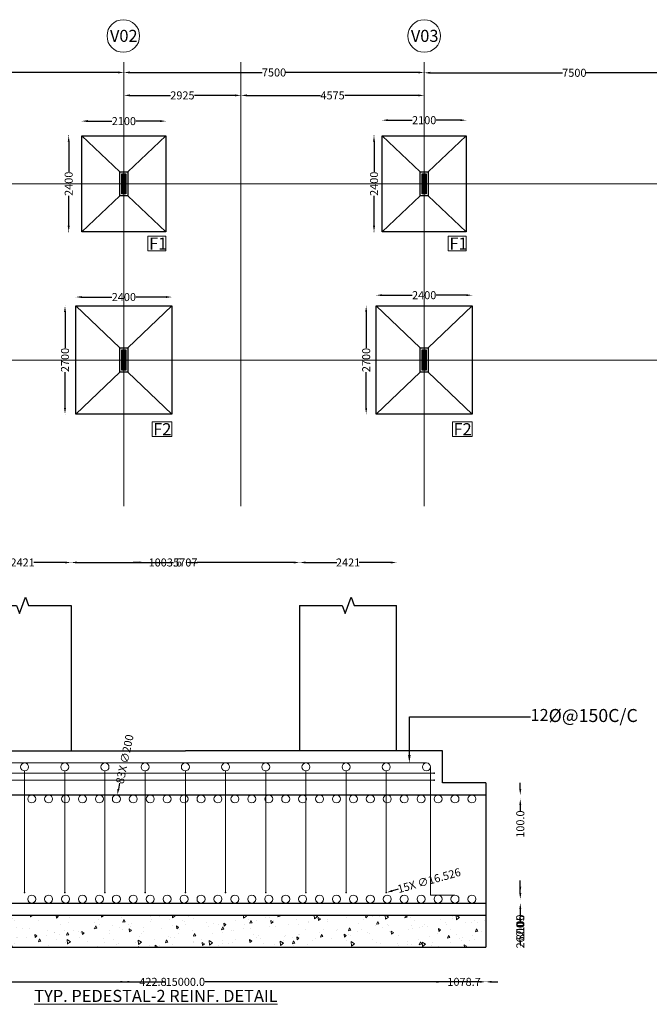
# Model space of a CAD drawing. Units: millimetres. Extents: x -30630 to 20484, y 3580 to 30715.
# Tile 2 of 4: x -19082 to -3358, y 3580 to 28161. Entities that reach past the tile are written whole.
import ezdxf
from ezdxf import colors
from ezdxf.entities.mleader import LeaderData, LeaderLine
from ezdxf.math import Vec2, Vec3

# ---------------------------------------------------------------- set-up
doc = ezdxf.new("R2010")
doc.units = ezdxf.units.MM
doc.header["$MEASUREMENT"] = 0
for name, color, linetype, lineweight in [('S-ANNO-DIMS', 2, 'Continuous', 18), ('S-ANNO-SYMB', 3, 'Continuous', 18), ('S-ANNO-TEXT', 7, 'Continuous', 18), ('S-CONC', 7, 'Continuous', 25), ('S-FNDN', 7, 'Continuous', 30), ('S-FNDN-PATT', 8, 'Continuous', 13), ('S-GRID', 1, 'Continuous', 18), ('S-GRID-IDEN', 7, 'Continuous', 18), ('S-REIN', 1, 'Continuous', 18)]:
    doc.layers.add(name, color=color, linetype=linetype, lineweight=lineweight)
doc.styles.get("Standard").update_dxf_attribs({"font": 'arial.ttf'})
doc.dimstyles.get("Standard").update_dxf_attribs({"dimtxt": 200, "dimasz": 150, "dimexe": 0.18, "dimexo": 0.0625, "dimgap": 0.09, "dimtad": 0, "dimdec": 0, "dimzin": 0, "dimdsep": 46, "dimtxsty": 'Standard', "dimcen": 0.09, "dimadec": 0, "dimazin": 0, "dimtfac": 1, "dimtdec": 0, "dimtofl": 0, "dimtmove": 0, "dimatfit": 3, "dimfxl": 1, "dimfxlon": 1, "dimtolj": 1, "dimtzin": 0, "dimarcsym": 0})

# ---------------------------------------------------------------- blocks, each defined once
blk = doc.blocks.new('*D1')
at = {"layer": 'Defpoints', "color": 0, "transparency": 16777216}
for p in [(-16480, 26844), (-23980, 25951), (-16480, 25951)]:
    blk.add_point(p, dxfattribs=at)
at = {"layer": 'S-ANNO-DIMS', "color": 0, "lineweight": -2, "transparency": 16777216}
for p, q in [((-23980, 26843), (-23980, 26844)), ((-23830, 26844), (-20528, 26844)), ((-16630, 26844), (-19933, 26844)), ((-16480, 26843), (-16480, 26844))]:
    blk.add_line(p, q, dxfattribs=at)
at = {"layer": 'S-ANNO-DIMS', "color": 0, "transparency": 16777216}
for points in [[(-23830, 26869), (-23830, 26819), (-23980, 26844)], [(-16630, 26869), (-16630, 26819), (-16480, 26844)]]:
    blk.add_solid(points, dxfattribs=at)
at = {"layer": 'S-ANNO-DIMS', "color": 0, "transparency": 16777216, "insert": (-20230, 26844), "char_height": 200, "attachment_point": 5}
blk.add_mtext('\\A1;7500', dxfattribs=at)
blk = doc.blocks.new('*D2')
at = {"layer": 'Defpoints', "color": 0, "transparency": 16777216}
for p in [(-16480, 26234), (-13555, 26271), (-13555, 26234)]:
    blk.add_point(p, dxfattribs=at)
at = {"layer": 'S-ANNO-DIMS', "color": 0, "lineweight": -2, "transparency": 16777216}
for p, q in [((-16480, 26270), (-16480, 26272)), ((-16330, 26271), (-15319, 26271)), ((-13705, 26271), (-14716, 26271)), ((-13555, 26270), (-13555, 26272))]:
    blk.add_line(p, q, dxfattribs=at)
at = {"layer": 'S-ANNO-DIMS', "color": 0, "transparency": 16777216}
for points in [[(-16330, 26296), (-16330, 26246), (-16480, 26271)], [(-13705, 26296), (-13705, 26246), (-13555, 26271)]]:
    blk.add_solid(points, dxfattribs=at)
at = {"layer": 'S-ANNO-DIMS', "color": 0, "transparency": 16777216, "insert": (-15018, 26271), "char_height": 200, "attachment_point": 5}
blk.add_mtext('\\A1;2925', dxfattribs=at)
blk = doc.blocks.new('*D3')
at = {"layer": 'Defpoints', "color": 0, "transparency": 16777216}
for p in [(-13555, 26271), (-8980, 26271), (-8980, 26271)]:
    blk.add_point(p, dxfattribs=at)
at = {"layer": 'S-ANNO-DIMS', "color": 0, "lineweight": -2, "transparency": 16777216}
for p, q in [((-13555, 26271), (-13555, 26271)), ((-13405, 26271), (-11571, 26271)), ((-9130, 26271), (-10964, 26271)), ((-8980, 26271), (-8980, 26271))]:
    blk.add_line(p, q, dxfattribs=at)
at = {"layer": 'S-ANNO-DIMS', "color": 0, "transparency": 16777216}
for points in [[(-13405, 26296), (-13405, 26246), (-13555, 26271)], [(-9130, 26296), (-9130, 26246), (-8980, 26271)]]:
    blk.add_solid(points, dxfattribs=at)
at = {"layer": 'S-ANNO-DIMS', "color": 0, "transparency": 16777216, "insert": (-11268, 26271), "char_height": 200, "attachment_point": 5}
blk.add_mtext('\\A1;4575', dxfattribs=at)
blk = doc.blocks.new('*D4')
at = {"layer": 'Defpoints', "color": 0, "transparency": 16777216}
for p in [(-16480, 26889), (-16480, 26843), (-8980, 26889)]:
    blk.add_point(p, dxfattribs=at)
at = {"layer": 'S-ANNO-DIMS', "color": 0, "lineweight": -2, "transparency": 16777216}
for p, q in [((-16480, 26844), (-16480, 26843)), ((-16330, 26843), (-13028, 26843)), ((-9130, 26843), (-12433, 26843)), ((-8980, 26844), (-8980, 26843))]:
    blk.add_line(p, q, dxfattribs=at)
at = {"layer": 'S-ANNO-DIMS', "color": 0, "transparency": 16777216}
for points in [[(-16330, 26868), (-16330, 26818), (-16480, 26843)], [(-9130, 26868), (-9130, 26818), (-8980, 26843)]]:
    blk.add_solid(points, dxfattribs=at)
at = {"layer": 'S-ANNO-DIMS', "color": 0, "transparency": 16777216, "insert": (-12730, 26843), "char_height": 200, "attachment_point": 5}
blk.add_mtext('\\A1;7500', dxfattribs=at)
blk = doc.blocks.new('*D5')
at = {"layer": 'Defpoints', "color": 0, "transparency": 16777216}
for p in [(-8980, 26835), (-8980, 26552), (-1480, 26552)]:
    blk.add_point(p, dxfattribs=at)
at = {"layer": 'S-ANNO-DIMS', "color": 0, "lineweight": -2, "transparency": 16777216}
for p, q in [((-8980, 26834), (-8980, 26836)), ((-8830, 26835), (-5528, 26835)), ((-1630, 26835), (-4933, 26835)), ((-1480, 26834), (-1480, 26836))]:
    blk.add_line(p, q, dxfattribs=at)
at = {"layer": 'S-ANNO-DIMS', "color": 0, "transparency": 16777216}
for points in [[(-8830, 26860), (-8830, 26810), (-8980, 26835)], [(-1630, 26860), (-1630, 26810), (-1480, 26835)]]:
    blk.add_solid(points, dxfattribs=at)
at = {"layer": 'S-ANNO-DIMS', "color": 0, "transparency": 16777216, "insert": (-5230, 26835), "char_height": 200, "attachment_point": 5}
blk.add_mtext('\\A1;7500', dxfattribs=at)
blk = doc.blocks.new('*D10')
at = {"layer": 'Defpoints', "color": 0, "transparency": 16777216}
for p in [(-15430, 25629), (-17530, 25265), (-15430, 25265)]:
    blk.add_point(p, dxfattribs=at)
at = {"layer": 'S-ANNO-DIMS', "color": 0, "lineweight": -2, "transparency": 16777216}
for p, q in [((-17530, 25628), (-17530, 25629)), ((-17380, 25629), (-16780, 25629)), ((-15580, 25629), (-16180, 25629)), ((-15430, 25628), (-15430, 25629))]:
    blk.add_line(p, q, dxfattribs=at)
at = {"layer": 'S-ANNO-DIMS', "color": 0, "transparency": 16777216}
for points in [[(-17380, 25654), (-17380, 25604), (-17530, 25629)], [(-15580, 25654), (-15580, 25604), (-15430, 25629)]]:
    blk.add_solid(points, dxfattribs=at)
at = {"layer": 'S-ANNO-DIMS', "color": 0, "transparency": 16777216, "insert": (-16480, 25629), "char_height": 200, "attachment_point": 5}
blk.add_mtext('\\A1;2100', dxfattribs=at)
blk = doc.blocks.new('*D11')
at = {"layer": 'Defpoints', "color": 0, "transparency": 16777216}
for p in [(-17530, 25265), (-17858, 22865), (-17530, 22865)]:
    blk.add_point(p, dxfattribs=at)
at = {"layer": 'S-ANNO-DIMS', "color": 0, "lineweight": -2, "transparency": 16777216}
for p, q in [((-17857, 25265), (-17859, 25265)), ((-17858, 25115), (-17858, 24365)), ((-17858, 23015), (-17858, 23765)), ((-17857, 22865), (-17859, 22865))]:
    blk.add_line(p, q, dxfattribs=at)
at = {"layer": 'S-ANNO-DIMS', "color": 0, "transparency": 16777216}
for points in [[(-17883, 25115), (-17833, 25115), (-17858, 25265)], [(-17883, 23015), (-17833, 23015), (-17858, 22865)]]:
    blk.add_solid(points, dxfattribs=at)
at = {"layer": 'S-ANNO-DIMS', "color": 0, "transparency": 16777216, "insert": (-17858, 24065), "char_height": 200, "attachment_point": 5, "rotation": 90}
blk.add_mtext('\\A1;2400', dxfattribs=at)
blk = doc.blocks.new('*D12')
at = {"layer": 'Defpoints', "color": 0, "transparency": 16777216}
for p in [(-7930, 25652), (-10030, 25265), (-7930, 25265)]:
    blk.add_point(p, dxfattribs=at)
at = {"layer": 'S-ANNO-DIMS', "color": 0, "lineweight": -2, "transparency": 16777216}
for p, q in [((-10030, 25651), (-10030, 25652)), ((-9880, 25652), (-9280, 25652)), ((-8080, 25652), (-8680, 25652)), ((-7930, 25651), (-7930, 25652))]:
    blk.add_line(p, q, dxfattribs=at)
at = {"layer": 'S-ANNO-DIMS', "color": 0, "transparency": 16777216}
for points in [[(-9880, 25677), (-9880, 25627), (-10030, 25652)], [(-8080, 25677), (-8080, 25627), (-7930, 25652)]]:
    blk.add_solid(points, dxfattribs=at)
at = {"layer": 'S-ANNO-DIMS', "color": 0, "transparency": 16777216, "insert": (-8980, 25652), "char_height": 200, "attachment_point": 5}
blk.add_mtext('\\A1;2100', dxfattribs=at)
blk = doc.blocks.new('*D13')
at = {"layer": 'Defpoints', "color": 0, "transparency": 16777216}
for p in [(-10030, 25265), (-10233, 22865), (-10030, 22865)]:
    blk.add_point(p, dxfattribs=at)
at = {"layer": 'S-ANNO-DIMS', "color": 0, "lineweight": -2, "transparency": 16777216}
for p, q in [((-10232, 25265), (-10234, 25265)), ((-10233, 25115), (-10233, 24365)), ((-10233, 23015), (-10233, 23765)), ((-10232, 22865), (-10234, 22865))]:
    blk.add_line(p, q, dxfattribs=at)
at = {"layer": 'S-ANNO-DIMS', "color": 0, "transparency": 16777216}
for points in [[(-10258, 25115), (-10208, 25115), (-10233, 25265)], [(-10258, 23015), (-10208, 23015), (-10233, 22865)]]:
    blk.add_solid(points, dxfattribs=at)
at = {"layer": 'S-ANNO-DIMS', "color": 0, "transparency": 16777216, "insert": (-10233, 24065), "char_height": 200, "attachment_point": 5, "rotation": 90}
blk.add_mtext('\\A1;2400', dxfattribs=at)
blk = doc.blocks.new('*D22')
at = {"layer": 'Defpoints', "color": 0, "transparency": 16777216}
for p in [(-17680, 21237), (-17680, 21015), (-15280, 21015)]:
    blk.add_point(p, dxfattribs=at)
at = {"layer": 'S-ANNO-DIMS', "color": 0, "lineweight": -2, "transparency": 16777216}
for p, q in [((-17680, 21236), (-17680, 21237)), ((-17530, 21237), (-16780, 21237)), ((-15430, 21237), (-16180, 21237)), ((-15280, 21236), (-15280, 21237))]:
    blk.add_line(p, q, dxfattribs=at)
at = {"layer": 'S-ANNO-DIMS', "color": 0, "transparency": 16777216}
for points in [[(-17530, 21262), (-17530, 21212), (-17680, 21237)], [(-15430, 21262), (-15430, 21212), (-15280, 21237)]]:
    blk.add_solid(points, dxfattribs=at)
at = {"layer": 'S-ANNO-DIMS', "color": 0, "transparency": 16777216, "insert": (-16480, 21237), "char_height": 200, "attachment_point": 5}
blk.add_mtext('\\A1;2400', dxfattribs=at)
blk = doc.blocks.new('*D23')
at = {"layer": 'Defpoints', "color": 0, "transparency": 16777216}
for p in [(-17680, 21015), (-17950, 18315), (-17680, 18315)]:
    blk.add_point(p, dxfattribs=at)
at = {"layer": 'S-ANNO-DIMS', "color": 0, "lineweight": -2, "transparency": 16777216}
for p, q in [((-17949, 21015), (-17950, 21015)), ((-17950, 20865), (-17950, 19965)), ((-17950, 18465), (-17950, 19365)), ((-17949, 18315), (-17950, 18315))]:
    blk.add_line(p, q, dxfattribs=at)
at = {"layer": 'S-ANNO-DIMS', "color": 0, "transparency": 16777216}
for points in [[(-17975, 20865), (-17925, 20865), (-17950, 21015)], [(-17975, 18465), (-17925, 18465), (-17950, 18315)]]:
    blk.add_solid(points, dxfattribs=at)
at = {"layer": 'S-ANNO-DIMS', "color": 0, "transparency": 16777216, "insert": (-17950, 19665), "char_height": 200, "attachment_point": 5, "rotation": 90}
blk.add_mtext('\\A1;2700', dxfattribs=at)
blk = doc.blocks.new('*D24')
at = {"layer": 'Defpoints', "color": 0, "transparency": 16777216}
for p in [(-10180, 21283), (-10180, 21015), (-7780, 21015)]:
    blk.add_point(p, dxfattribs=at)
at = {"layer": 'S-ANNO-DIMS', "color": 0, "lineweight": -2, "transparency": 16777216}
for p, q in [((-10180, 21282), (-10180, 21283)), ((-10030, 21283), (-9280, 21283)), ((-7930, 21283), (-8680, 21283)), ((-7780, 21282), (-7780, 21283))]:
    blk.add_line(p, q, dxfattribs=at)
at = {"layer": 'S-ANNO-DIMS', "color": 0, "transparency": 16777216}
for points in [[(-10030, 21308), (-10030, 21258), (-10180, 21283)], [(-7930, 21308), (-7930, 21258), (-7780, 21283)]]:
    blk.add_solid(points, dxfattribs=at)
at = {"layer": 'S-ANNO-DIMS', "color": 0, "transparency": 16777216, "insert": (-8980, 21283), "char_height": 200, "attachment_point": 5}
blk.add_mtext('\\A1;2400', dxfattribs=at)
blk = doc.blocks.new('*D25')
at = {"layer": 'Defpoints', "color": 0, "transparency": 16777216}
for p in [(-10180, 21015), (-10429, 18315), (-10180, 18315)]:
    blk.add_point(p, dxfattribs=at)
at = {"layer": 'S-ANNO-DIMS', "color": 0, "lineweight": -2, "transparency": 16777216}
for p, q in [((-10428, 21015), (-10429, 21015)), ((-10429, 20865), (-10429, 19965)), ((-10429, 18465), (-10429, 19365)), ((-10428, 18315), (-10429, 18315))]:
    blk.add_line(p, q, dxfattribs=at)
at = {"layer": 'S-ANNO-DIMS', "color": 0, "transparency": 16777216}
for points in [[(-10454, 20865), (-10404, 20865), (-10429, 21015)], [(-10454, 18465), (-10404, 18465), (-10429, 18315)]]:
    blk.add_solid(points, dxfattribs=at)
at = {"layer": 'S-ANNO-DIMS', "color": 0, "transparency": 16777216, "insert": (-10429, 19665), "char_height": 200, "attachment_point": 5, "rotation": 90}
blk.add_mtext('\\A1;2700', dxfattribs=at)
blk = doc.blocks.new('FOOTING-F1')
h = blk.add_hatch()
h.set_pattern_fill('ANSI31', color=256, scale=100)
h.set_pattern_definition([(45, (50626.339, 2179.544), (-8.8388348, 8.8388348), [])])
h.paths.add_polyline_path([(1100, 24315), (1000, 24315), (1000, 23815), (1100, 23815)])
for p, q in [((0, 25265), (950, 24365)), ((1150, 24365), (2100, 25265)), ((950, 23765), (0, 22865)), ((1150, 23765), (2100, 22865))]:
    blk.add_line(p, q)
for points in [[(0, 25265), (2100, 25265), (2100, 22865), (0, 22865)], [(950, 24365), (1150, 24365), (1150, 23765), (950, 23765)], [(1000, 24315), (1100, 24315), (1100, 23815), (1000, 23815)]]:
    blk.add_lwpolyline(points, close=True)
blk = doc.blocks.new('FOOTING-F2')
h = blk.add_hatch()
h.set_pattern_fill('ANSI31', color=256, scale=100)
h.set_pattern_definition([(45, (58801.161, 2265.705), (-8.8388348, 8.8388348), [])])
h.paths.add_polyline_path([(1250, 19915), (1150, 19915), (1150, 19415), (1250, 19415)])
for p, q in [((1100, 19965), (0, 21015)), ((1300, 19965), (2400, 21015)), ((1100, 19365), (0, 18315)), ((1300, 19365), (2400, 18315))]:
    blk.add_line(p, q)
for points in [[(0, 21015), (2400, 21015), (2400, 18315), (0, 18315)], [(1100, 19965), (1300, 19965), (1300, 19365), (1100, 19365)], [(1150, 19915), (1250, 19915), (1250, 19415), (1150, 19415)]]:
    blk.add_lwpolyline(points, close=True)
blk = doc.blocks.new('*D36')
at = {"layer": 'Defpoints', "color": 0, "transparency": 16777216}
for p in [(-7445, 5806), (-6580, 5806), (-7445, 5006)]:
    blk.add_point(p, dxfattribs=at)
at = {"layer": 'S-ANNO-DIMS', "color": 0, "lineweight": -2, "transparency": 16777216}
for p, q in [((-6581, 5806), (-6580, 5806)), ((-6580, 5656), (-6580, 5627)), ((-6580, 5156), (-6580, 5186)), ((-6581, 5006), (-6580, 5006))]:
    blk.add_line(p, q, dxfattribs=at)
at = {"layer": 'S-ANNO-DIMS', "color": 0, "transparency": 16777216}
for points in [[(-6605, 5656), (-6555, 5656), (-6580, 5806)], [(-6605, 5156), (-6555, 5156), (-6580, 5006)]]:
    blk.add_solid(points, dxfattribs=at)
at = {"layer": 'S-ANNO-DIMS', "color": 0, "transparency": 16777216, "insert": (-6580, 5406), "char_height": 200, "attachment_point": 5, "rotation": 90}
blk.add_mtext('\\A1;800', dxfattribs=at)
blk = doc.blocks.new('*D40')
at = {"layer": 'Defpoints', "color": 0, "transparency": 16777216}
for p in [(-23310, 13539), (-12091, 13539), (-12091, 9906)]:
    blk.add_point(p, dxfattribs=at)
at = {"layer": 'S-ANNO-DIMS', "color": 0, "lineweight": -2, "transparency": 16777216}
for p, q in [((-23309, 13539), (-23310, 13539)), ((-23310, 13389), (-23310, 12021)), ((-23310, 10056), (-23310, 11424)), ((-23309, 9906), (-23310, 9906))]:
    blk.add_line(p, q, dxfattribs=at)
at = {"layer": 'S-ANNO-DIMS', "color": 0, "transparency": 16777216}
for points in [[(-23335, 13389), (-23285, 13389), (-23310, 13539)], [(-23335, 10056), (-23285, 10056), (-23310, 9906)]]:
    blk.add_solid(points, dxfattribs=at)
at = {"layer": 'S-ANNO-DIMS', "color": 0, "transparency": 16777216, "insert": (-23310, 11723), "char_height": 200, "attachment_point": 5, "rotation": 90}
blk.add_mtext('\\A1;3633', dxfattribs=at)
blk = doc.blocks.new('*D42')
at = {"layer": 'Defpoints', "color": 0, "transparency": 16777216}
for p in [(-8523, 9106), (-7445, 9106), (-7445, 4141)]:
    blk.add_point(p, dxfattribs=at)
at = {"layer": 'S-ANNO-DIMS', "color": 0, "lineweight": -2, "transparency": 16777216}
for p, q in [((-8673, 4141), (-8823, 4141)), ((-8523, 4142), (-8523, 4141)), ((-7445, 4142), (-7445, 4141)), ((-7295, 4141), (-7145, 4141))]:
    blk.add_line(p, q, dxfattribs=at)
at = {"layer": 'S-ANNO-DIMS', "color": 0, "transparency": 16777216}
for points in [[(-8673, 4166), (-8673, 4116), (-8523, 4141)], [(-7295, 4166), (-7295, 4116), (-7445, 4141)]]:
    blk.add_solid(points, dxfattribs=at)
at = {"layer": 'S-ANNO-DIMS', "color": 0, "transparency": 16777216, "insert": (-7984, 4141), "char_height": 200, "attachment_point": 5}
blk.add_mtext('\\A1;1078.7', dxfattribs=at)
blk = doc.blocks.new('*D43')
at = {"layer": 'Defpoints', "color": 0, "transparency": 16777216}
for p in [(-17798, 14610), (-20219, 13539), (-17798, 13539)]:
    blk.add_point(p, dxfattribs=at)
at = {"layer": 'S-ANNO-DIMS', "color": 0, "lineweight": -2, "transparency": 16777216}
for p, q in [((-20219, 14609), (-20219, 14611)), ((-20069, 14610), (-19290, 14610)), ((-17948, 14610), (-18727, 14610)), ((-17798, 14609), (-17798, 14611))]:
    blk.add_line(p, q, dxfattribs=at)
at = {"layer": 'S-ANNO-DIMS', "color": 0, "transparency": 16777216}
for points in [[(-20069, 14635), (-20069, 14585), (-20219, 14610)], [(-17948, 14635), (-17948, 14585), (-17798, 14610)]]:
    blk.add_solid(points, dxfattribs=at)
at = {"layer": 'S-ANNO-DIMS', "color": 0, "transparency": 16777216, "insert": (-19009, 14610), "char_height": 200, "attachment_point": 5}
blk.add_mtext('\\A1;2421', dxfattribs=at)
blk = doc.blocks.new('*D44')
at = {"layer": 'Defpoints', "color": 0, "transparency": 16777216}
for p in [(-12091, 14610), (-17798, 13539), (-12091, 13539)]:
    blk.add_point(p, dxfattribs=at)
at = {"layer": 'S-ANNO-DIMS', "color": 0, "lineweight": -2, "transparency": 16777216}
for p, q in [((-17798, 14609), (-17798, 14611)), ((-17648, 14610), (-15243, 14610)), ((-12241, 14610), (-14646, 14610)), ((-12091, 14609), (-12091, 14611))]:
    blk.add_line(p, q, dxfattribs=at)
at = {"layer": 'S-ANNO-DIMS', "color": 0, "transparency": 16777216}
for points in [[(-17648, 14635), (-17648, 14585), (-17798, 14610)], [(-12241, 14635), (-12241, 14585), (-12091, 14610)]]:
    blk.add_solid(points, dxfattribs=at)
at = {"layer": 'S-ANNO-DIMS', "color": 0, "transparency": 16777216, "insert": (-14945, 14610), "char_height": 200, "attachment_point": 5}
blk.add_mtext('\\A1;5707', dxfattribs=at)
blk = doc.blocks.new('*D45')
at = {"layer": 'Defpoints', "color": 0, "transparency": 16777216}
for p in [(-9670, 14610), (-12091, 13539), (-9670, 13539)]:
    blk.add_point(p, dxfattribs=at)
at = {"layer": 'S-ANNO-DIMS', "color": 0, "lineweight": -2, "transparency": 16777216}
for p, q in [((-12091, 14609), (-12091, 14611)), ((-11941, 14610), (-11162, 14610)), ((-9820, 14610), (-10600, 14610)), ((-9670, 14609), (-9670, 14611))]:
    blk.add_line(p, q, dxfattribs=at)
at = {"layer": 'S-ANNO-DIMS', "color": 0, "transparency": 16777216}
for points in [[(-11941, 14635), (-11941, 14585), (-12091, 14610)], [(-9820, 14635), (-9820, 14585), (-9670, 14610)]]:
    blk.add_solid(points, dxfattribs=at)
at = {"layer": 'S-ANNO-DIMS', "color": 0, "transparency": 16777216, "insert": (-10881, 14610), "char_height": 200, "attachment_point": 5}
blk.add_mtext('\\A1;2421', dxfattribs=at)
blk = doc.blocks.new('*D46')
at = {"layer": 'Defpoints', "color": 0, "transparency": 16777216}
for p in [(-16668, 6206), (-16245, 6206), (-16245, 4141)]:
    blk.add_point(p, dxfattribs=at)
at = {"layer": 'S-ANNO-DIMS', "color": 0, "lineweight": -2, "transparency": 16777216}
for p, q in [((-16668, 4142), (-16668, 4141)), ((-16518, 4141), (-16395, 4141)), ((-16245, 4142), (-16245, 4141)), ((-16245, 4141), (-16095, 4141))]:
    blk.add_line(p, q, dxfattribs=at)
at = {"layer": 'S-ANNO-DIMS', "color": 0, "transparency": 16777216}
for points in [[(-16518, 4166), (-16518, 4116), (-16668, 4141)], [(-16395, 4166), (-16395, 4116), (-16245, 4141)]]:
    blk.add_solid(points, dxfattribs=at)
at = {"layer": 'S-ANNO-DIMS', "color": 0, "transparency": 16777216, "insert": (-15753, 4141), "char_height": 200, "attachment_point": 5}
blk.add_mtext('\\A1;422.8', dxfattribs=at)
blk = doc.blocks.new('*D47')
at = {"layer": 'Defpoints', "color": 0, "transparency": 16777216}
for p in [(-14944.743439, 14610.362834), (-15948.299713, 9506.371523), (-14944.743439, 9506.371523)]:
    blk.add_point(p, dxfattribs=at)
at = {"layer": 'S-ANNO-DIMS', "color": 0, "lineweight": -2, "transparency": 16777216}
for p, q in [((-16098.299713, 14610.362834), (-16248.299713, 14610.362834)), ((-15948.299713, 14609.362834), (-15948.299713, 14610.542834)), ((-14944.743439, 14609.362834), (-14944.743439, 14610.542834)), ((-14794.743439, 14610.362834), (-14644.743439, 14610.362834))]:
    blk.add_line(p, q, dxfattribs=at)
at = {"layer": 'S-ANNO-DIMS', "color": 0, "transparency": 16777216}
for points in [[(-16098.299713, 14635.362834), (-16098.299713, 14585.362834), (-15948.299713, 14610.362834)], [(-14794.743439, 14635.362834), (-14794.743439, 14585.362834), (-14944.743439, 14610.362834)]]:
    blk.add_solid(points, dxfattribs=at)
at = {"layer": 'S-ANNO-DIMS', "color": 0, "transparency": 16777216, "insert": (-15446.521576, 14610.362834), "char_height": 200, "attachment_point": 5}
blk.add_mtext('\\A1;1003.6', dxfattribs=at)
blk = doc.blocks.new('*D48')
at = {"layer": 'Defpoints', "color": 0, "transparency": 16777216}
for p in [(-7788, 6206), (-7445, 6106), (-6580, 6106)]:
    blk.add_point(p, dxfattribs=at)
at = {"layer": 'S-ANNO-DIMS', "color": 0, "lineweight": -2, "transparency": 16777216}
for p, q in [((-6580, 6356), (-6580, 6506)), ((-6581, 6206), (-6580, 6206)), ((-6581, 6106), (-6580, 6106)), ((-6580, 5956), (-6580, 5806))]:
    blk.add_line(p, q, dxfattribs=at)
at = {"layer": 'S-ANNO-DIMS', "color": 0, "transparency": 16777216}
for points in [[(-6605, 6356), (-6555, 6356), (-6580, 6206)], [(-6605, 5956), (-6555, 5956), (-6580, 6106)]]:
    blk.add_solid(points, dxfattribs=at)
at = {"layer": 'S-ANNO-DIMS', "color": 0, "transparency": 16777216, "insert": (-6580, 5595), "char_height": 200, "attachment_point": 5, "rotation": 90}
blk.add_mtext('\\A1;100', dxfattribs=at)
blk = doc.blocks.new('*D60')
at = {"layer": 'Defpoints', "color": 0, "transparency": 16777216}
for p in [(-16688, 8608), (-16647, 8804)]:
    blk.add_point(p, dxfattribs=at)
at = {"layer": 'S-ANNO-DIMS', "color": 0, "lineweight": -2, "transparency": 16777216}
for p, q in [((-16586, 9098), (-16617, 8951)), ((-16668, 8706), (-16668, 8706)), ((-16668, 8706), (-16668, 8706))]:
    blk.add_line(p, q, dxfattribs=at)
at = {"layer": 'S-ANNO-DIMS', "color": 0, "transparency": 16777216}
blk.add_solid([(-16641, 8956), (-16592, 8946), (-16647, 8804)], dxfattribs=at)
at = {"layer": 'S-ANNO-DIMS', "color": 0, "transparency": 16777216, "insert": (-16460, 9702), "char_height": 200, "attachment_point": 5, "rotation": 78.23}
blk.add_mtext('\\A1;83X ∅200', dxfattribs=at)
blk = doc.blocks.new('*D65')
at = {"layer": 'Defpoints', "color": 0, "transparency": 16777216}
for p in [(-23880, 24365), (-23880, 23765), (19772, 23765)]:
    blk.add_point(p, dxfattribs=at)
at = {"layer": 'S-ANNO-DIMS', "color": 0, "lineweight": -2, "transparency": 16777216}
for p, q in [((19771, 24365), (19772, 24365)), ((19772, 24215), (19772, 23915)), ((19771, 23765), (19772, 23765)), ((19772, 23765), (19772, 23615))]:
    blk.add_line(p, q, dxfattribs=at)
at = {"layer": 'S-ANNO-DIMS', "color": 0, "transparency": 16777216}
for points in [[(19747, 24215), (19797, 24215), (19772, 24365)], [(19747, 23915), (19797, 23915), (19772, 23765)]]:
    blk.add_solid(points, dxfattribs=at)
at = {"layer": 'S-ANNO-DIMS', "color": 0, "transparency": 16777216, "insert": (19772, 23277), "char_height": 200, "attachment_point": 5, "rotation": 90}
blk.add_mtext('\\A1;600.0', dxfattribs=at)
blk = doc.blocks.new('*D68')
at = {"layer": 'Defpoints', "color": 0, "transparency": 16777216}
for p in [(-22445, 6106), (-7445, 6106), (-7445, 4141)]:
    blk.add_point(p, dxfattribs=at)
at = {"layer": 'S-ANNO-DIMS', "color": 0, "lineweight": -2, "transparency": 16777216}
for p, q in [((-22445, 4142), (-22445, 4141)), ((-22295, 4141), (-15428, 4141)), ((-7595, 4141), (-14462, 4141)), ((-7445, 4142), (-7445, 4141))]:
    blk.add_line(p, q, dxfattribs=at)
at = {"layer": 'S-ANNO-DIMS', "color": 0, "transparency": 16777216}
for points in [[(-22295, 4166), (-22295, 4116), (-22445, 4141)], [(-7595, 4166), (-7595, 4116), (-7445, 4141)]]:
    blk.add_solid(points, dxfattribs=at)
at = {"layer": 'S-ANNO-DIMS', "color": 0, "transparency": 16777216, "insert": (-14945, 4141), "char_height": 200, "attachment_point": 5}
blk.add_mtext('\\A1;15000.0', dxfattribs=at)
blk = doc.blocks.new('*D70')
at = {"layer": 'Defpoints', "color": 0, "transparency": 16777216}
for p in [(-7788, 8706), (-7445, 8806), (-6580, 8706)]:
    blk.add_point(p, dxfattribs=at)
at = {"layer": 'S-ANNO-DIMS', "color": 0, "lineweight": -2, "transparency": 16777216}
for p, q in [((-6580, 8956), (-6580, 9106)), ((-6581, 8806), (-6580, 8806)), ((-6581, 8706), (-6580, 8706)), ((-6580, 8556), (-6580, 8406))]:
    blk.add_line(p, q, dxfattribs=at)
at = {"layer": 'S-ANNO-DIMS', "color": 0, "transparency": 16777216}
for points in [[(-6605, 8956), (-6555, 8956), (-6580, 8806)], [(-6605, 8556), (-6555, 8556), (-6580, 8706)]]:
    blk.add_solid(points, dxfattribs=at)
at = {"layer": 'S-ANNO-DIMS', "color": 0, "transparency": 16777216, "insert": (-6580, 8079), "char_height": 200, "attachment_point": 5, "rotation": 90}
blk.add_mtext('\\A1;100.0', dxfattribs=at)
blk = doc.blocks.new('*D72')
at = {"layer": 'Defpoints', "color": 0, "transparency": 16777216}
for p in [(-9927, 6370), (-9922, 6108), (-6580, 6108)]:
    blk.add_point(p, dxfattribs=at)
at = {"layer": 'S-ANNO-DIMS', "color": 0, "lineweight": -2, "transparency": 16777216}
for p, q in [((-6580, 6520), (-6580, 6670)), ((-6581, 6370), (-6580, 6370)), ((-6581, 6108), (-6580, 6108)), ((-6580, 5958), (-6580, 5808))]:
    blk.add_line(p, q, dxfattribs=at)
at = {"layer": 'S-ANNO-DIMS', "color": 0, "transparency": 16777216}
for points in [[(-6605, 6520), (-6555, 6520), (-6580, 6370)], [(-6605, 5958), (-6555, 5958), (-6580, 6108)]]:
    blk.add_solid(points, dxfattribs=at)
at = {"layer": 'S-ANNO-DIMS', "color": 0, "transparency": 16777216, "insert": (-6580, 5391), "char_height": 200, "attachment_point": 5, "rotation": 90}
blk.add_mtext('\\A1;262.05', dxfattribs=at)
blk = doc.blocks.new('*D81')
at = {"layer": 'Defpoints', "color": 0, "transparency": 16777216}
for p in [(-9935, 6368), (-9919, 6373)]:
    blk.add_point(p, dxfattribs=at)
at = {"layer": 'S-ANNO-DIMS', "color": 0, "lineweight": -2, "transparency": 16777216}
for p, q in [((-9630, 6454), (-9775, 6413)), ((-9927, 6370), (-9927, 6371)), ((-9927, 6370), (-9927, 6370))]:
    blk.add_line(p, q, dxfattribs=at)
at = {"layer": 'S-ANNO-DIMS', "color": 0, "transparency": 16777216}
blk.add_solid([(-9781, 6437), (-9768, 6389), (-9919, 6373)], dxfattribs=at)
at = {"layer": 'S-ANNO-DIMS', "color": 0, "transparency": 16777216, "insert": (-8858, 6671), "char_height": 200, "attachment_point": 5, "rotation": 15.6897}
blk.add_mtext('\\A1;15X ∅16.526', dxfattribs=at)

msp = doc.modelspace()

# ---------------------------------------------------------------- hatches: boundary and pattern name
at = {"layer": 'S-FNDN-PATT'}
h = msp.add_hatch(dxfattribs=at)
h.set_pattern_fill('AR-CONC', color=256, scale=100, angle=47)
h.set_pattern_definition([(97, (-6254.7, 5540.77), (535.064, 481.774), [75, -825]), (42, (-6254.7, 5540.8), (-644.747, 411.518), [60, -660]), (147.4514, (-6210.1, 5580.9), (-109.682, 893.292), [63.74, -701.142]), (93.184, (-6401, 5677.2), (848.91, 667.647), [112.5, -1237.5]), (143.636, (-6330.2, 5732.8), (-74.99, 1347.916), [95.61, -1051.714]), (38.184, (-6401, 5677.2), (-74.99, 1347.916), [90, -990]), (68, (-6296.2, 5716.2), (701.546, 161.965), [75, -825]), (13, (-6296.2, 5716.2), (-364.4, 672.5), [60, -660]), (118.4514, (-6237.74, 5729.7), (337.146, 834.465), [63.74, -701.142]), (84.5, (-6254.7, 5540.77), (-235.17, 235.9262), [0, -652, 0, -670, 0, -662.5]), (54.5, (-6254.7, 5540.77), (-109.0415, 461.385), [0, -382, 0, -637, 0, -252.5]), (14.5, (-6406.8, 5377.67), (380.5616, 375.0306), [0, -250, 0, -780, 0, -1035]), (4.5, (-6475, 5304.54), (324.52, 494.787), [0, -325, 0, -518, 0, -735])])
h.paths.add_polyline_path([(-7444.7434, 5006.3715), (-7444.7434, 5806.3715), (-22444.7434, 5806.3715), (-22444.7434, 5006.3715)])

# ---------------------------------------------------------------- linework, layer by layer
at = {"layer": 'S-ANNO-SYMB'}
for points in [[(-15880.1095, 22391.7904), (-15880.1095, 22753.0183), (-15430.0685, 22753.0183), (-15430.0685, 22391.7904)], [(-8380.1095, 22391.7904), (-8380.1095, 22753.0183), (-7930.0685, 22753.0183), (-7930.0685, 22391.7904)], [(-15777.1763, 17757.175), (-15777.1763, 18118.4029), (-15280.0685, 18118.4029), (-15280.0685, 17757.175)], [(-8277.1763, 17757.175), (-8277.1763, 18118.4029), (-7780.0685, 18118.4029), (-7780.0685, 17757.175)]]:
    msp.add_lwpolyline(points, close=True, dxfattribs=at)
at = {"layer": 'S-CONC'}
for p, q in [((-17798.1943, 13539.302), (-17798.1943, 9906.3715)), ((-12091.2926, 13539.302), (-12091.2926, 9906.3715)), ((-9670.3306, 9906.3715), (-9670.3306, 13539.302)), ((-21366.0811, 9906.3715), (-14944.7434, 9906.3715)), ((-8523.4058, 9906.3715), (-14944.7434, 9906.3715)), ((-8523.4058, 9106.3715), (-8523.4058, 9906.3715)), ((-7444.7434, 9106.3715), (-8523.4058, 9106.3715)), ((-7444.7434, 9106.3715), (-7444.7434, 5806.3715)), ((-22444.7434, 8806.3715), (-7444.7434, 8806.3715)), ((-22444.7434, 6106.3715), (-7444.7434, 6106.3715)), ((-22444.7434, 5806.3715), (-7444.7434, 5806.3715)), ((-7444.7434, 5806.3715), (-7444.7434, 5006.3715)), ((-22444.7434, 5006.3715), (-7444.7434, 5006.3715))]:
    msp.add_line(p, q, dxfattribs=at)
for points in [[(-20219.3363, 13539.302), (-19158.6753, 13539.302), (-19083.6753, 13333.2412), (-18933.6753, 13745.3628), (-18858.6753, 13539.302), (-17798.0143, 13539.302)], [(-12091.4726, 13539.302), (-11030.8116, 13539.302), (-10955.8116, 13333.2412), (-10805.8116, 13745.3628), (-10730.8116, 13539.302), (-9670.1506, 13539.302)]]:
    msp.add_lwpolyline(points, dxfattribs=at)
at = {"layer": 'S-GRID'}
for p, q in [((-16480.0685, 27102.0571), (-16480.0685, 16015.6561)), ((-13555.0685, 27102.0571), (-13555.0685, 16015.6561)), ((-8980.0685, 27102.0571), (-8980.0685, 16015.6561)), ((-26695.8159, 24064.7195), (17349.3354, 24064.7195)), ((-26695.8159, 19664.7195), (17349.3354, 19664.7195))]:
    msp.add_line(p, q, dxfattribs=at)
at = {"layer": 'S-GRID-IDEN'}
for centre in [(-16493.7641, 27753.8802), (-8980.0685, 27753.8802)]:
    msp.add_circle(centre, 407.0061, dxfattribs=at)
at = {"layer": 'S-REIN'}
for p, q in [((-20966.0811, 9606.3715), (-14944.7434, 9606.3715)), ((-8923.4058, 9606.3715), (-14944.7434, 9606.3715)), ((-21140.5094, 9349.192), (-8740.6319, 9349.192)), ((-18958.9685, 9406.3715), (-18958.9685, 6378.7119)), ((-17955.4123, 9406.3715), (-17955.4123, 6378.7119)), ((-16951.856, 9406.3715), (-16951.856, 6378.7119)), ((-15948.2997, 9406.3715), (-15948.2997, 6378.7119)), ((-14944.7434, 9406.3715), (-14944.7434, 6378.7119)), ((-13941.1872, 9406.3715), (-13941.1872, 6378.7119)), ((-12937.6309, 9406.3715), (-12937.6309, 6378.7119)), ((-11934.0746, 9406.3715), (-11934.0746, 6378.7119)), ((-10930.5183, 9406.3715), (-10930.5183, 6378.7119)), ((-9926.9621, 9406.3715), (-9926.9621, 6378.7119)), ((-8823.4058, 9106.3715), (-8823.4058, 9506.3715)), ((-21140.5094, 9174.6041), (-8740.6319, 9174.6041)), ((-8823.4058, 9106.3715), (-8823.4058, 6306.3715)), ((-8823.4058, 6306.3715), (-8210.9654, 6306.3715))]:
    msp.add_line(p, q, dxfattribs=at)
for centre, radius in [((-18958.9685, 9506.3715), 100), ((-17955.4123, 9506.3715), 100), ((-16951.856, 9506.3715), 100), ((-15948.2997, 9506.3715), 100), ((-14944.7434, 9506.3715), 100), ((-13941.1872, 9506.3715), 100), ((-12937.6309, 9506.3715), 100), ((-11934.0746, 9506.3715), 100), ((-10930.5183, 9506.3715), 100), ((-9926.9621, 9506.3715), 100), ((-8923.4058, 9506.3715), 100), ((-8732.3688, 9349.192), 8.263), ((-8732.3688, 9174.6041), 8.263), ((-18781.9575, 8706.3715), 100), ((-18359.1178, 8706.3715), 100), ((-17936.2781, 8706.3715), 100), ((-17513.4384, 8706.3715), 100), ((-17090.5987, 8706.3715), 100), ((-16667.7591, 8706.3715), 100), ((-16244.9194, 8706.3715), 100), ((-15822.0797, 8706.3715), 100), ((-15399.24, 8706.3715), 100), ((-14976.4003, 8706.3715), 100), ((-14553.5607, 8706.3715), 100), ((-14130.721, 8706.3715), 100), ((-13707.8813, 8706.3715), 100), ((-13285.0416, 8706.3715), 100), ((-12862.2019, 8706.3715), 100), ((-12439.3622, 8706.3715), 100), ((-12016.5226, 8706.3715), 100), ((-11593.6829, 8706.3715), 100), ((-11170.8432, 8706.3715), 100), ((-10748.0035, 8706.3715), 100), ((-10325.1638, 8706.3715), 100), ((-9902.3242, 8706.3715), 100), ((-9479.4845, 8706.3715), 100), ((-9056.6448, 8706.3715), 100), ((-8633.8051, 8706.3715), 100), ((-8210.9654, 8706.3715), 100), ((-7788.1257, 8706.3715), 100), ((-18958.9685, 6370.4489), 8.263), ((-18781.9575, 6206.3715), 100), ((-18359.1178, 6206.3715), 100), ((-17936.2781, 6206.3715), 100), ((-17955.4123, 6370.4489), 8.263), ((-17513.4384, 6206.3715), 100), ((-17090.5987, 6206.3715), 100), ((-16951.856, 6370.4489), 8.263), ((-16667.7591, 6206.3715), 100), ((-16244.9194, 6206.3715), 100), ((-15948.2997, 6370.4489), 8.263), ((-15822.0797, 6206.3715), 100), ((-15399.24, 6206.3715), 100), ((-14976.4003, 6206.3715), 100), ((-14944.7434, 6370.4489), 8.263), ((-14553.5607, 6206.3715), 100), ((-14130.721, 6206.3715), 100), ((-13941.1872, 6370.4489), 8.263), ((-13707.8813, 6206.3715), 100), ((-13285.0416, 6206.3715), 100), ((-12862.2019, 6206.3715), 100), ((-12937.6309, 6370.4489), 8.263), ((-12439.3622, 6206.3715), 100), ((-12016.5226, 6206.3715), 100), ((-11934.0746, 6370.4489), 8.263), ((-11593.6829, 6206.3715), 100), ((-11170.8432, 6206.3715), 100), ((-10930.5183, 6370.4489), 8.263), ((-10748.0035, 6206.3715), 100), ((-10325.1638, 6206.3715), 100), ((-9902.3242, 6206.3715), 100), ((-9926.9621, 6370.4489), 8.263), ((-9479.4845, 6206.3715), 100), ((-9056.6448, 6206.3715), 100), ((-8633.8051, 6206.3715), 100), ((-8210.9654, 6206.3715), 100), ((-7788.1257, 6206.3715), 100)]:
    msp.add_circle(centre, radius, dxfattribs=at)

# ---------------------------------------------------------------- block references
at = {"layer": 'S-FNDN'}
for name, p in [('FOOTING-F1', (-17530.069, 0)), ('FOOTING-F1', (-10030.069, 0)), ('FOOTING-F2', (-17680.069, 0)), ('FOOTING-F2', (-10180.069, 0))]:
    msp.add_blockref(name, p, dxfattribs=at)

# ---------------------------------------------------------------- texts
at = {"layer": 'S-ANNO-TEXT', "char_height": 300, "attachment_point": 1}
for s, width, insert in [('V02', 4876.019723, (-16827.2225, 27907.0521)), ('V03', 4876.019723, (-9313.5269, 27907.0521)), ('{\\fArial|b1|i0|c0|p34;F1}', 1058.385802, (-15850.1095, 22723.0183)), ('{\\fArial|b1|i0|c0|p34;F1}', 1058.385802, (-8350.1095, 22723.0183)), ('{\\fArial|b1|i0|c0|p34;F2}', 1058.385802, (-15747.1763, 18088.4029)), ('{\\fArial|b1|i0|c0|p34;F2}', 1058.385802, (-8247.1763, 18088.4029)), ('{\\fArial|b1|i0|c0|p34;\\LTYP. PEDESTAL-2 REINF. DETAIL}', 7568.651815, (-18717.7533, 3940.2472))]:
    msp.add_mtext_dynamic_manual_height_columns(s, width=width, gutter_width=1, heights=[0], dxfattribs=dict(at, insert=insert))

# ---------------------------------------------------------------- dimensions: what is measured, and where the dimension line sits
at = {"layer": 'S-ANNO-DIMS'}
for base, p1, p2, override, picture, middle in [((-16480.0685, 26843.6702), (-23980.0685, 25950.8365), (-16480.0685, 25950.8365), {"dimclrd": 0, "dimclre": 0, "dimclrt": 0}, '*D1', (-20230.0685, 26843.6702)), ((-16480.0685, 26843.2602), (-8980.0685, 26889.1319), (-16480.0685, 26889.1319), {"dimclrd": 0, "dimclre": 0, "dimclrt": 0}, '*D4', (-12730.0685, 26843.2602)), ((-8980.0685, 26835.3937), (-1480.0685, 26552.1998), (-8980.0685, 26552.1998), {"dimclrd": 0, "dimclre": 0, "dimclrt": 0}, '*D5', (-5230.0685, 26835.3937)), ((-13555.0685, 26271.47), (-16480.0685, 26233.9285), (-13555.0685, 26233.9285), {"dimclrd": 0, "dimclre": 0, "dimclrt": 0}, '*D2', (-15017.5685, 26271.47)), ((-8980.0685, 26271.06), (-13555.0685, 26271.06), (-8980.0685, 26271.06), {"dimclrd": 0, "dimclre": 0, "dimclrt": 0}, '*D3', (-11267.5685, 26271.06)), ((-15430.0685, 25629.0271), (-17530.0685, 25264.7195), (-15430.0685, 25264.7195), {"dimclrd": 0, "dimclre": 0, "dimclrt": 0}, '*D10', (-16480.0685, 25629.0271)), ((-7930.0685, 25651.9681), (-10030.0685, 25264.7195), (-7930.0685, 25264.7195), {"dimclrd": 0, "dimclre": 0, "dimclrt": 0}, '*D12', (-8980.0685, 25651.9681)), ((-10180.0685, 21282.5519), (-7780.0685, 21014.7195), (-10180.0685, 21014.7195), {"dimclrd": 0, "dimclre": 0, "dimclrt": 0}, '*D24', (-8980.0685, 21282.5519)), ((-17680.0685, 21236.8254), (-15280.0685, 21014.7195), (-17680.0685, 21014.7195), {"dimclrd": 0, "dimclre": 0, "dimclrt": 0}, '*D22', (-16480.0685, 21236.8254)), ((-17798.0143, 14610.3628), (-20219.1563, 13539.302), (-17798.0143, 13539.302), {"dimdec": 0, "dimlfac": 1, "dimrnd": 0, "dimzin": 0, "dimdsep": 46, "dimlunit": 2}, '*D43', (-19008.5853, 14610.3628)), ((-12091.2926, 14610.3628), (-17798.0143, 13539.302), (-12091.2926, 13539.302), {"dimdec": 0, "dimlfac": 1, "dimrnd": 0, "dimzin": 0, "dimdsep": 46, "dimlunit": 2}, '*D44', (-14944.6534, 14610.3628)), ((-14944.7434, 14610.3628), (-15948.2997, 9506.3715), (-14944.7434, 9506.3715), {"dimdec": 1, "dimlfac": 1, "dimrnd": 0, "dimzin": 0, "dimdsep": 46, "dimlunit": 2}, '*D47', (-15446.5216, 14610.3628)), ((-9670.1506, 14610.3628), (-12091.2926, 13539.302), (-9670.1506, 13539.302), {"dimdec": 0, "dimlfac": 1, "dimrnd": 0, "dimzin": 0, "dimdsep": 46, "dimlunit": 2}, '*D45', (-10880.7216, 14610.3628)), ((-7444.7434, 4141.3715), (-8523.4058, 9106.3715), (-7444.7434, 9106.3715), {"dimdec": 1, "dimlfac": 1, "dimrnd": 0, "dimzin": 0, "dimdsep": 46, "dimlunit": 2}, '*D42', (-7984.0746, 4141.3715)), ((-16244.9194, 4141.3715), (-16667.7591, 6206.3715), (-16244.9194, 6206.3715), {"dimdec": 1, "dimlfac": 1, "dimrnd": 0, "dimzin": 0, "dimdsep": 46, "dimlunit": 2}, '*D46', (-15753.1513, 4141.3715)), ((-7444.7434, 4141.3715), (-22444.7434, 6106.3715), (-7444.7434, 6106.3715), {"dimdec": 1, "dimlfac": 1, "dimrnd": 0, "dimzin": 0, "dimdsep": 46, "dimlunit": 2}, '*D68', (-14944.7434, 4141.3715))]:
    dim = msp.add_linear_dim(base=base, p1=p1, p2=p2, dimstyle='Standard', override=override, dxfattribs=at)
    dim.commit()
    dim.dimension.update_dxf_attribs({"geometry": picture, "text_midpoint": middle})
for base, p1, p2, override, picture, middle in [((-17858.4181, 22864.7195), (-17530.0685, 25264.7195), (-17530.0685, 22864.7195), {"dimclrd": 0, "dimclre": 0, "dimclrt": 0}, '*D11', (-17858.4181, 24064.7195)), ((-10233.4673, 22864.7195), (-10030.0685, 25264.7195), (-10030.0685, 22864.7195), {"dimclrd": 0, "dimclre": 0, "dimclrt": 0}, '*D13', (-10233.4673, 24064.7195)), ((19771.8354, 23764.7195), (-23880.0685, 24364.7195), (-23880.0685, 23764.7195), {"dimdec": 1, "dimlfac": 1, "dimrnd": 0, "dimzin": 0, "dimdsep": 46, "dimlunit": 2}, '*D65', (19771.8354, 23276.976)), ((-17949.8232, 18314.7195), (-17680.0685, 21014.7195), (-17680.0685, 18314.7195), {"dimclrd": 0, "dimclre": 0, "dimclrt": 0}, '*D23', (-17949.8232, 19664.7195)), ((-10429.1511, 18314.7195), (-10180.0685, 21014.7195), (-10180.0685, 18314.7195), {"dimclrd": 0, "dimclre": 0, "dimclrt": 0}, '*D25', (-10429.1511, 19664.7195)), ((-23309.7434, 13539.302), (-12091.2926, 9906.3715), (-12091.2926, 13539.302), {"dimdec": 0, "dimlfac": 1, "dimrnd": 0, "dimzin": 0, "dimdsep": 46, "dimlunit": 2}, '*D40', (-23309.7434, 11722.8368)), ((-6579.7434, 8706.3715), (-7444.7434, 8806.3715), (-7788.1257, 8706.3715), {"dimdec": 1, "dimlfac": 1, "dimrnd": 0, "dimzin": 0, "dimdsep": 46, "dimlunit": 2}, '*D70', (-6579.7434, 8078.5871)), ((-6579.7434, 6108.4032), (-9926.9621, 6370.4489), (-9922.4776, 6108.4032), {"dimdec": 2, "dimlfac": 1, "dimrnd": 0, "dimzin": 0, "dimdsep": 46, "dimlunit": 2}, '*D72', (-6579.7434, 5390.7143)), ((-6579.7434, 6106.3715), (-7788.1257, 6206.3715), (-7444.7434, 6106.3715), {"dimdec": 0, "dimlfac": 1, "dimrnd": 0, "dimzin": 0, "dimdsep": 46, "dimlunit": 2}, '*D48', (-6579.7434, 5595.0946)), ((-6579.7434, 5806.3715), (-7444.7434, 5006.3715), (-7444.7434, 5806.3715), {"dimdec": 0, "dimlfac": 1, "dimrnd": 0, "dimzin": 0, "dimdsep": 46, "dimlunit": 2}, '*D36', (-6579.7434, 5406.3715))]:
    dim = msp.add_linear_dim(base=base, p1=p1, p2=p2, angle=90, dimstyle='Standard', override=override, dxfattribs=at)
    dim.commit()
    dim.dimension.update_dxf_attribs({"geometry": picture, "text_midpoint": middle})
for p1, p2, text, override, picture, middle in [((-16688.1574, 8608.4741), (-16647.3607, 8804.269), '83X <>', {"dimdec": 0, "dimlfac": 1, "dimrnd": 0, "dimzin": 0, "dimdsep": 46, "dimlunit": 2}, '*D60', (-16460.334, 9701.8614)), ((-9934.9172, 6368.2143), (-9919.0069, 6372.6834), '15X <>', {"dimdec": 3, "dimlfac": 1, "dimrnd": 0, "dimzin": 0, "dimdsep": 46, "dimlunit": 2}, '*D81', (-8858.264, 6670.6388))]:
    dim = msp.add_diameter_dim_2p(p1=p1, p2=p2, text=text, dimstyle='Standard', override=override, dxfattribs=at)
    dim.commit()
    dim.dimension.update_dxf_attribs({"geometry": picture, "text_midpoint": middle, "dimtype": 163})

# ---------------------------------------------------------------- leaders
at = {"layer": 'S-ANNO-TEXT'}
ml = msp.add_multileader_mtext('Standard', dxfattribs=at)
ml.set_content('12{\\H1.08333x;Ø@150C/C}', color=256)
ml.set_leader_properties()
ml.build(insert=Vec2(0, 0))
ml.multileader.update_dxf_attribs({"dogleg_length": 0.36, "arrow_head_size": 200})
ctx = ml.context
ctx.base_point, ctx.char_height, ctx.arrow_head_size, ctx.landing_gap_size, ctx.plane_origin = Vec3(-6326.4066, 10754.6775), 300, 200, 0.09, Vec3(-9350.0448, 9606.3715)
notes = []
notes.append((ctx, [(0, (1, 1, 0), (-6326.7666, 10754.6775), (1, 0), 0.36, [(0, [(-9350.0448, 9606.3715), (-9350.0448, 10754.6775)], 0, [])])]))
ctx.mtext.insert, ctx.mtext.width, ctx.mtext.flow_direction = Vec3(-6326.3166, 10952.4519), 2458.179759, 5
for ctx, leaders in notes:
    for number, flags, end, landing, length, lines in leaders:
        leader = LeaderData()
        leader.index, (leader.has_last_leader_line, leader.has_dogleg_vector, leader.attachment_direction) = number, flags
        leader.last_leader_point, leader.dogleg_vector, leader.dogleg_length = Vec3(end), Vec3(landing), length
        for number, points, colour, breaks in lines:
            line = LeaderLine()
            line.index, line.vertices, line.color, line.breaks = number, Vec3.list(points), colors.encode_raw_color(colour), breaks
            leader.lines.append(line)
        ctx.leaders.append(leader)

doc.saveas('drawing.dxf')
